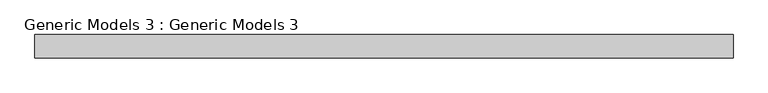
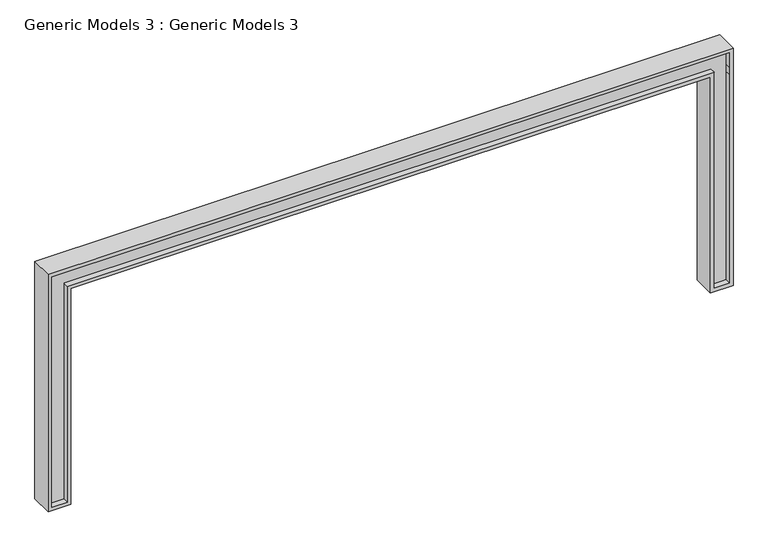
"""IFC4 building model written with IfcOpenShell, lengths in millimetres: proxy geometry, Generic Models 3 : Generic Models 3."""

from ifc_helpers import new_model, si_unit, origin, place, context, project, spatial, faceted_brep, source, transform, mapped, element, save


def generic_models_3_generic_models_3_9b1755e3(model_context):
    return source(origin(), model_context, "Body", "Brep", [
        faceted_brep([(589.554407, -4416.274389, 3352.8), (589.554407, -4416.274389, 0.0), (894.354407, -4416.274389, 0.0), (894.354407, -4416.274389, 3048.0), (9428.754407, -4416.274389, 3048.0), (9428.754407, -4416.274389, 0.0), (9733.554407, -4416.274389, 0.0), (9733.554407, -4416.274389, 3352.8), (9479.554407, -4416.274389, 50.8), (9479.554407, -4416.274389, 3098.8), (843.554407, -4416.274389, 3098.8), (843.554407, -4416.274389, 50.8), (640.354407, -4416.274389, 50.8), (640.354407, -4416.274389, 2997.2), (640.354407, -4416.274389, 3098.8), (640.354407, -4416.274389, 3302.0), (9682.754407, -4416.274389, 3302.0), (9682.754407, -4416.274389, 3098.8), (9682.754407, -4416.274389, 2997.2), (9682.754407, -4416.274389, 50.8), (589.554407, -4111.474389, 3352.8), (9733.554407, -4111.474389, 3352.8), (9733.554407, -4111.474389, 0.0), (9428.754407, -4111.474389, 0.0), (9428.754407, -4111.474389, 3048.0), (894.354407, -4111.474389, 3048.0), (894.354407, -4111.474389, 0.0), (589.554407, -4111.474389, 0.0), (9479.554407, -4111.474389, 3098.8), (9479.554407, -4111.474389, 50.8), (9682.754407, -4111.474389, 50.8), (9682.754407, -4111.474389, 3302.0), (640.354407, -4111.474389, 3302.0), (640.354407, -4111.474389, 50.8), (843.554407, -4111.474389, 50.8), (843.554407, -4111.474389, 3098.8), (9479.554407, -4146.6030678, 3098.8), (9479.554407, -4146.6030678, 50.8), (843.554407, -4146.6030678, 3098.8), (843.554407, -4146.6030678, 50.8), (640.354407, -4146.6030678, 50.8), (640.354407, -4146.6030678, 3302.0), (9682.754407, -4146.6030678, 3302.0), (9682.754407, -4146.6030678, 50.8), (9479.554407, -4340.074389, 50.8), (9682.754407, -4340.074389, 50.8), (9682.754407, -4340.074389, 2997.2), (9682.754407, -4340.074389, 3098.8), (9682.754407, -4340.074389, 3302.0), (640.354407, -4340.074389, 3302.0), (640.354407, -4340.074389, 3098.8), (640.354407, -4340.074389, 2997.2), (640.354407, -4340.074389, 50.8), (843.554407, -4340.074389, 50.8), (843.554407, -4340.074389, 3098.8), (9479.554407, -4340.074389, 3098.8)], [[[0, 1, 2, 3, 4, 5, 6, 7], [8, 9, 10, 11, 12, 13, 14, 15, 16, 17, 18, 19]], [[20, 21, 22, 23, 24, 25, 26, 27], [28, 29, 30, 31, 32, 33, 34, 35]], [[1, 0, 20, 27]], [[2, 1, 27, 26]], [[3, 2, 26, 25]], [[4, 3, 25, 24]], [[5, 4, 24, 23]], [[6, 5, 23, 22]], [[7, 6, 22, 21]], [[0, 7, 21, 20]], [[36, 37, 29, 28]], [[38, 36, 28, 35]], [[39, 38, 35, 34]], [[40, 39, 34, 33]], [[41, 40, 33, 32]], [[42, 41, 32, 31]], [[43, 42, 31, 30]], [[37, 43, 30, 29]], [[37, 36, 38, 39, 40, 41, 42, 43]], [[44, 45, 46, 47, 48, 49, 50, 51, 52, 53, 54, 55]], [[44, 55, 9, 8]], [[55, 54, 10, 9]], [[54, 53, 11, 10]], [[53, 52, 12, 11]], [[52, 51, 13, 12]], [[51, 50, 14, 13]], [[50, 49, 15, 14]], [[49, 48, 16, 15]], [[48, 47, 17, 16]], [[47, 46, 18, 17]], [[46, 45, 19, 18]], [[45, 44, 8, 19]]]),
    ])


if __name__ == "__main__":
    model = new_model("IFC4")
    model_context = context("Model", 3, world=origin())
    ifc_project = project(units=[si_unit("LENGTHUNIT", "METRE", prefix="MILLI")], contexts=[model_context])
    site = spatial("IfcSite", under=ifc_project)
    building = spatial("IfcBuilding", under=site)
    placement = place(None, origin())
    generic_models_3_generic_models_3_shape = generic_models_3_generic_models_3_9b1755e3(model_context)
    element("IfcBuildingElementProxy", 1, Name="Generic Models 3 : Generic Models 3", ObjectType="Generic Models 3 : Generic Models 3", at=placement, inside=building, context=model_context, shape_type="MappedRepresentation", body=[
        mapped(generic_models_3_generic_models_3_shape, transform((0.0, 0.0, 0.0), x_axis=(1.0, 0.0, 0.0), y_axis=(0.0, 1.0, 0.0), z_axis=(0.0, 0.0, 1.0))),
    ])
    save(model, "model.ifc")

# Revit data of these elements
# Element 1 (IfcBuildingElementProxy, "Generic Models 3 : Generic Models 3")
#   Materials on its faces: "LIGHT GREY WHITE", "Iron, Ductile"
# Materials
#   "LIGHT GREY WHITE": class "Generic", colour RGB 120 120 120, transparency 0, Cost = 0
#   "Iron, Ductile": class "Metal", colour RGB 0 0 0, transparency 0, Description = "Ductile cast iron", Cost = 0
